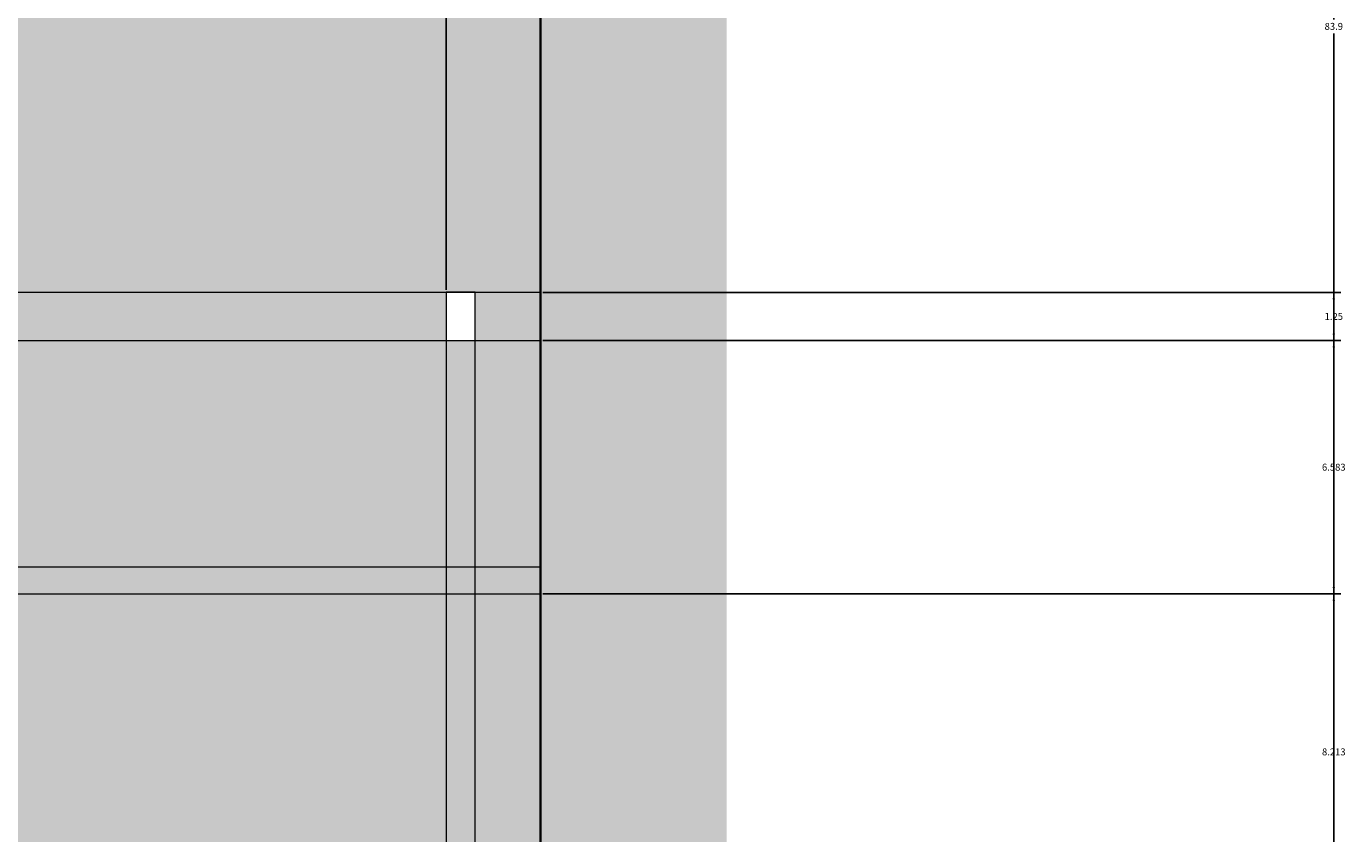
# Model space of a CAD drawing. Units: feet. Extents: x 2695 to 2912, y 795 to 1139.
# Tile 60 of 83: x 2877 to 2912, y 958 to 979. Entities that reach past the tile are written whole.
import ezdxf

# ---------------------------------------------------------------- set-up
doc = ezdxf.new("R2010")
doc.units = ezdxf.units.FT
for name, color, linetype, lineweight in [('A-ANNO-DIMS', 2, 'Continuous', 18), ('A-ELEV', 7, 'Continuous', 35), ('A-ELEV-PATT', 252, 'Continuous', 13), ('A-ELEV-RAIL', 8, 'Continuous', 18)]:
    doc.layers.add(name, color=color, linetype=linetype, lineweight=lineweight)
doc.styles.get("Standard").update_dxf_attribs({"font": 'arial.ttf'})
doc.dimstyles.get("Standard").update_dxf_attribs({"dimtxt": 0.18, "dimasz": 0.18, "dimexe": 0.18, "dimexo": 0.0625, "dimgap": 0.09, "dimtad": 0, "dimtih": 1, "dimtoh": 1, "dimdec": 1, "dimzin": 0, "dimdsep": 46, "dimlunit": 3, "dimtxsty": 'Standard', "dimcen": 0.09, "dimadec": 0, "dimazin": 0, "dimtfac": 1, "dimtdec": 1, "dimtofl": 0, "dimtmove": 0, "dimatfit": 3, "dimfxl": 1, "dimtolj": 1, "dimtzin": 0, "dimarcsym": 0})

# ---------------------------------------------------------------- blocks, each defined once
blk = doc.blocks.new('*D17')
at = {"layer": 'A-ANNO-DIMS', "color": 0, "lineweight": -2, "transparency": 16777216}
for p, q in [((2843.637, 1020.824), (2911.424, 1020.824)), ((2911.244, 1020.644), (2911.244, 979.059)), ((2911.244, 937.111), (2911.244, 978.695)), ((2890.699, 936.931), (2911.424, 936.931))]:
    blk.add_line(p, q, dxfattribs=at)
at = {"layer": 'A-ANNO-DIMS', "color": 0, "transparency": 16777216}
for points in [[(2911.214, 1020.644), (2911.274, 1020.644), (2911.244, 1020.824)], [(2911.214, 937.111), (2911.274, 937.111), (2911.244, 936.931)]]:
    blk.add_solid(points, dxfattribs=at)
at = {"layer": 'Defpoints', "color": 0, "transparency": 16777216}
for p in [(2843.575, 1020.824), (2911.244, 1020.824), (2890.636, 936.931)]:
    blk.add_point(p, dxfattribs=at)
at = {"layer": 'A-ANNO-DIMS', "color": 0, "transparency": 16777216, "insert": (2911.244, 978.877), "char_height": 0.18, "attachment_point": 5}
blk.add_mtext('\\A1;83.9', dxfattribs=at)
blk = doc.blocks.new('*D50')
at = {"layer": 'A-ANNO-DIMS', "color": 0, "lineweight": -2, "transparency": 16777216}
for p, q in [((2810.041, 972.03), (2810.041, 1138.886)), ((2888.188, 972.03), (2888.188, 1138.886)), ((2810.221, 1138.706), (2848.721, 1138.706)), ((2888.008, 1138.706), (2849.508, 1138.706))]:
    blk.add_line(p, q, dxfattribs=at)
at = {"layer": 'A-ANNO-DIMS', "color": 0, "transparency": 16777216}
for points in [[(2810.221, 1138.736), (2810.221, 1138.676), (2810.041, 1138.706)], [(2888.008, 1138.736), (2888.008, 1138.676), (2888.188, 1138.706)]]:
    blk.add_solid(points, dxfattribs=at)
at = {"layer": 'Defpoints', "color": 0, "transparency": 16777216}
for p in [(2888.188, 1138.706), (2810.041, 971.967), (2888.188, 971.967)]:
    blk.add_point(p, dxfattribs=at)
at = {"layer": 'A-ANNO-DIMS', "color": 0, "transparency": 16777216, "insert": (2849.114, 1138.706), "char_height": 0.18, "attachment_point": 5}
blk.add_mtext('\\A1;78.15', dxfattribs=at)
blk = doc.blocks.new('*D51')
at = {"layer": 'A-ANNO-DIMS', "color": 0, "lineweight": -2, "transparency": 16777216}
for p, q in [((2888.188, 972.03), (2888.188, 1138.886)), ((2890.636, 972.03), (2890.636, 1138.886)), ((2888.368, 1138.706), (2889.017, 1138.706)), ((2890.456, 1138.706), (2889.808, 1138.706))]:
    blk.add_line(p, q, dxfattribs=at)
at = {"layer": 'A-ANNO-DIMS', "color": 0, "transparency": 16777216}
for points in [[(2888.368, 1138.736), (2888.368, 1138.676), (2888.188, 1138.706)], [(2890.456, 1138.736), (2890.456, 1138.676), (2890.636, 1138.706)]]:
    blk.add_solid(points, dxfattribs=at)
at = {"layer": 'Defpoints', "color": 0, "transparency": 16777216}
for p in [(2890.636, 1138.706), (2888.188, 971.967), (2890.636, 971.967)]:
    blk.add_point(p, dxfattribs=at)
at = {"layer": 'A-ANNO-DIMS', "color": 0, "transparency": 16777216, "insert": (2889.412, 1138.706), "char_height": 0.18, "attachment_point": 5}
blk.add_mtext('\\A1;2.448', dxfattribs=at)
blk = doc.blocks.new('*D57')
at = {"layer": 'A-ANNO-DIMS', "color": 0, "lineweight": -2, "transparency": 16777216}
for p, q in [((2890.699, 964.133), (2911.424, 964.133)), ((2911.244, 963.953), (2911.244, 960.208)), ((2911.244, 956.1), (2911.244, 959.845)), ((2890.699, 955.92), (2911.424, 955.92))]:
    blk.add_line(p, q, dxfattribs=at)
at = {"layer": 'A-ANNO-DIMS', "color": 0, "transparency": 16777216}
for points in [[(2911.214, 963.953), (2911.274, 963.953), (2911.244, 964.133)], [(2911.214, 956.1), (2911.274, 956.1), (2911.244, 955.92)]]:
    blk.add_solid(points, dxfattribs=at)
at = {"layer": 'Defpoints', "color": 0, "transparency": 16777216}
for p in [(2890.636, 964.133), (2911.244, 964.133), (2890.636, 955.92)]:
    blk.add_point(p, dxfattribs=at)
at = {"layer": 'A-ANNO-DIMS', "color": 0, "transparency": 16777216, "insert": (2911.244, 960.027), "char_height": 0.18, "attachment_point": 5}
blk.add_mtext('\\A1;8.213', dxfattribs=at)
blk = doc.blocks.new('*D58')
at = {"layer": 'A-ANNO-DIMS', "color": 0, "lineweight": -2, "transparency": 16777216}
for p, q in [((2890.699, 970.716), (2911.424, 970.716)), ((2911.244, 970.536), (2911.244, 967.606)), ((2911.244, 964.313), (2911.244, 967.242)), ((2890.699, 964.133), (2911.424, 964.133))]:
    blk.add_line(p, q, dxfattribs=at)
at = {"layer": 'A-ANNO-DIMS', "color": 0, "transparency": 16777216}
for points in [[(2911.214, 970.536), (2911.274, 970.536), (2911.244, 970.716)], [(2911.214, 964.313), (2911.274, 964.313), (2911.244, 964.133)]]:
    blk.add_solid(points, dxfattribs=at)
at = {"layer": 'Defpoints', "color": 0, "transparency": 16777216}
for p in [(2890.636, 970.716), (2911.244, 970.716), (2890.636, 964.133)]:
    blk.add_point(p, dxfattribs=at)
at = {"layer": 'A-ANNO-DIMS', "color": 0, "transparency": 16777216, "insert": (2911.244, 967.424), "char_height": 0.18, "attachment_point": 5}
blk.add_mtext('\\A1;6.583', dxfattribs=at)
blk = doc.blocks.new('*D59')
at = {"layer": 'A-ANNO-DIMS', "color": 0, "lineweight": -2, "transparency": 16777216}
for p, q in [((2890.699, 971.967), (2911.424, 971.967)), ((2911.244, 971.787), (2911.244, 971.523)), ((2911.244, 970.896), (2911.244, 971.16)), ((2890.699, 970.716), (2911.424, 970.716))]:
    blk.add_line(p, q, dxfattribs=at)
at = {"layer": 'A-ANNO-DIMS', "color": 0, "transparency": 16777216}
for points in [[(2911.214, 971.787), (2911.274, 971.787), (2911.244, 971.967)], [(2911.214, 970.896), (2911.274, 970.896), (2911.244, 970.716)]]:
    blk.add_solid(points, dxfattribs=at)
at = {"layer": 'Defpoints', "color": 0, "transparency": 16777216}
for p in [(2890.636, 971.967), (2911.244, 971.967), (2890.636, 970.716)]:
    blk.add_point(p, dxfattribs=at)
at = {"layer": 'A-ANNO-DIMS', "color": 0, "transparency": 16777216, "insert": (2911.244, 971.341), "char_height": 0.18, "attachment_point": 5}
blk.add_mtext('\\A1;1.25', dxfattribs=at)

msp = doc.modelspace()

# ---------------------------------------------------------------- hatches: boundary and pattern name
at = {"layer": 'A-ELEV-PATT'}
h = msp.add_hatch(color=256, dxfattribs=at)
h.set_gradient(color1=(147, 149, 152), color2=(147, 149, 152), tint=1)
h.paths.add_polyline_path([(2770.6361, 1118.4096), (2710.6361, 1118.4096), (2710.6361, 1062.9306), (2770.6361, 1062.9306)])
h.paths.add_polyline_path([(2890.6361, 1103.3378), (2770.6361, 1103.3378), (2770.6361, 1062.9306), (2890.6361, 1062.9306)])
h.paths.add_polyline_path([(2730.7081, 1048.1052), (2755.1125, 1048.1052), (2755.1125, 936.9306), (2770.6361, 936.9306), (2770.6361, 1050.3105), (2715.8852, 1050.3105), (2715.8852, 936.9306), (2730.7081, 936.9306)])
h.paths.add_polyline_path([(2890.6361, 1050.3105), (2770.6361, 1050.3105), (2770.6361, 971.9673), (2778.0341, 971.9673), (2778.0341, 1020.8235), (2843.575, 1020.8235), (2843.575, 971.9673), (2890.6361, 971.9673)])
h.paths.add_polyline_path([(2888.1882, 970.7156), (2843.575, 970.7156), (2843.575, 964.8267), (2888.1882, 964.8267)])
h.paths.add_polyline_path([(2888.1882, 964.1328), (2843.575, 964.1328), (2843.575, 956.614), (2888.1882, 956.614)])
h.paths.add_polyline_path([(2888.1882, 955.9202), (2843.575, 955.9202), (2843.575, 949.2892), (2888.1882, 949.2892)])
h.paths.add_polyline_path([(2888.1882, 948.5954), (2843.575, 948.5954), (2843.575, 941.3507), (2888.1882, 941.3507)])
h.paths.add_polyline_path([(2888.1882, 940.6569), (2843.575, 940.6569), (2843.575, 936.9306), (2888.1882, 936.9306)])
h.paths.add_polyline_path([(2890.6361, 970.7156), (2888.9368, 970.7156), (2888.9368, 964.8267), (2890.6361, 964.8267)])
h.paths.add_polyline_path([(2890.6361, 964.1328), (2888.9368, 964.1328), (2888.9368, 956.614), (2890.6361, 956.614)])
h.paths.add_polyline_path([(2890.6361, 955.9202), (2888.9368, 955.9202), (2888.9368, 949.2892), (2890.6361, 949.2892)])
h.paths.add_polyline_path([(2890.6361, 940.6569), (2888.9368, 940.6569), (2888.9368, 936.9306), (2890.6361, 936.9306)])
h.paths.add_polyline_path([(2890.6361, 948.5954), (2888.9368, 948.5954), (2888.9368, 941.3507), (2890.6361, 941.3507)])
h.paths.add_polyline_path([(2772.5216, 970.7156), (2770.6361, 970.7156), (2770.6361, 964.8267), (2772.5216, 964.8267)])
h.paths.add_polyline_path([(2772.5216, 964.1328), (2770.6361, 964.1328), (2770.6361, 956.614), (2772.5216, 956.614)])
h.paths.add_polyline_path([(2772.5216, 955.9202), (2770.6361, 955.9202), (2770.6361, 949.2892), (2772.5216, 949.2892)])
h.paths.add_polyline_path([(2772.5216, 948.5954), (2770.6361, 948.5954), (2770.6361, 941.3507), (2772.5216, 941.3507)])
h.paths.add_polyline_path([(2772.5216, 940.6569), (2770.6361, 940.6569), (2770.6361, 936.9306), (2772.5216, 936.9306)])
h.paths.add_polyline_path([(2778.0341, 940.6569), (2773.2702, 940.6569), (2773.2702, 936.9306), (2778.0341, 936.9306)])
h.paths.add_polyline_path([(2778.0341, 970.7156), (2773.2702, 970.7156), (2773.2702, 964.8267), (2778.0341, 964.8267)])
h.paths.add_polyline_path([(2778.0341, 964.1328), (2773.2702, 964.1328), (2773.2702, 956.614), (2778.0341, 956.614)])
h.paths.add_polyline_path([(2778.0341, 955.9202), (2773.2702, 955.9202), (2773.2702, 949.2892), (2778.0341, 949.2892)])
h.paths.add_polyline_path([(2778.0341, 948.5954), (2773.2702, 948.5954), (2773.2702, 941.3507), (2778.0341, 941.3507)])
h.paths.add_polyline_path([(2810.0407, 940.6569), (2780.0341, 940.6569), (2780.0341, 936.9306), (2810.0407, 936.9306)])
h.paths.add_polyline_path([(2890.6361, 924.3105), (2770.6361, 924.3105), (2770.6361, 810.9306), (2773.5029, 810.9306), (2773.5029, 905.5143), (2805.9398, 905.5143), (2838.3767, 905.5143), (2838.3767, 810.9306), (2890.6361, 810.9306)])
h = msp.add_hatch(color=256, dxfattribs=at)
h.set_gradient(color1=(255, 255, 255), tint=1)
h.paths.add_polyline_path([(2895.4694, 1107.8588), (2890.6361, 1107.8588), (2890.6361, 810.9306), (2895.4694, 810.9306)])
h = msp.add_hatch(color=256, dxfattribs=at)
h.set_gradient(color1=(255, 255, 255), tint=1)
h.paths.add_polyline_path([(2890.6361, 1050.3105), (2881.9484, 1050.3105), (2881.9484, 971.9673), (2890.6361, 971.9673)])
h.paths.add_polyline_path([(2888.1882, 970.7156), (2881.9484, 970.7156), (2881.9484, 964.8267), (2888.1882, 964.8267)])
h.paths.add_polyline_path([(2890.6361, 970.7156), (2888.9368, 970.7156), (2888.9368, 964.8267), (2890.6361, 964.8267)])
h.paths.add_polyline_path([(2888.1882, 964.1328), (2881.9484, 964.1328), (2881.9484, 956.614), (2888.1882, 956.614)])
h.paths.add_polyline_path([(2890.6361, 964.1328), (2888.9368, 964.1328), (2888.9368, 956.614), (2890.6361, 956.614)])
h.paths.add_polyline_path([(2888.1882, 955.9202), (2881.9484, 955.9202), (2881.9484, 949.2892), (2888.1882, 949.2892)])
h.paths.add_polyline_path([(2890.6361, 955.9202), (2888.9368, 955.9202), (2888.9368, 949.2892), (2890.6361, 949.2892)])
h.paths.add_polyline_path([(2888.1882, 948.5954), (2881.9484, 948.5954), (2881.9484, 941.3507), (2888.1882, 941.3507)])
h.paths.add_polyline_path([(2890.6361, 948.5954), (2888.9368, 948.5954), (2888.9368, 941.3507), (2890.6361, 941.3507)])
h.paths.add_polyline_path([(2888.1882, 940.6569), (2881.9484, 940.6569), (2881.9484, 936.9306), (2888.1882, 936.9306)])
h = msp.add_hatch(color=256, dxfattribs=at)
h.set_gradient(color2=(0, 0, 0), tint=1)
h.paths.add_polyline_path([(2772.5216, 971.9673), (2770.6361, 971.9673), (2770.6361, 970.7156), (2772.5216, 970.7156)])
h.paths.add_polyline_path([(2773.2702, 971.9673), (2772.5216, 971.9673), (2772.5216, 970.7156), (2773.2702, 970.7156)])
h.paths.add_polyline_path([(2778.0341, 971.9673), (2773.2702, 971.9673), (2773.2702, 970.7156), (2778.0341, 970.7156)])
h.paths.add_polyline_path([(2780.0341, 971.9673), (2778.0341, 971.9673), (2778.0341, 970.7156), (2780.0341, 970.7156)])
h.paths.add_polyline_path([(2841.575, 971.9673), (2780.0341, 971.9673), (2780.0341, 970.7156), (2841.575, 970.7156)])
h.paths.add_polyline_path([(2843.575, 971.9673), (2841.575, 971.9673), (2841.575, 970.7156), (2843.575, 970.7156)])
h.paths.add_polyline_path([(2888.1882, 971.9673), (2843.575, 971.9673), (2843.575, 970.7156), (2888.1882, 970.7156)])
h.paths.add_polyline_path([(2888.9368, 971.9673), (2888.1882, 971.9673), (2888.1882, 970.7156), (2888.9368, 970.7156)], flags=17)
h.paths.add_polyline_path([(2890.6361, 971.9673), (2888.9368, 971.9673), (2888.9368, 970.7156), (2890.6361, 970.7156)])
h.paths.add_polyline_path([(2888.9368, 971.9673), (2888.1882, 971.9673), (2888.1882, 964.8267), (2888.9368, 964.8267)])
h.paths.add_polyline_path([(2888.9368, 964.8267), (2888.1882, 964.8267), (2888.1882, 964.1328), (2888.9368, 964.1328)])
h.paths.add_polyline_path([(2890.6361, 964.8267), (2888.9368, 964.8267), (2888.9368, 964.1328), (2890.6361, 964.1328)])
h.paths.add_polyline_path([(2888.1882, 964.8267), (2770.6361, 964.8267), (2770.6361, 964.1328), (2888.1882, 964.1328)])
h.paths.add_polyline_path([(2888.9368, 964.1328), (2888.1882, 964.1328), (2888.1882, 936.9306), (2888.9368, 936.9306)])
h.paths.add_polyline_path([(2890.6361, 956.614), (2888.9368, 956.614), (2888.9368, 955.9202), (2890.6361, 955.9202)])
h.paths.add_polyline_path([(2888.1882, 956.614), (2770.6361, 956.614), (2770.6361, 955.9202), (2888.1882, 955.9202)])
h.paths.add_polyline_path([(2890.6361, 949.2892), (2888.9368, 949.2892), (2888.9368, 948.5954), (2890.6361, 948.5954)])
h.paths.add_polyline_path([(2888.1882, 949.2892), (2770.6361, 949.2892), (2770.6361, 948.5954), (2888.1882, 948.5954)])
h.paths.add_polyline_path([(2890.6361, 941.3507), (2888.9368, 941.3507), (2888.9368, 940.6569), (2890.6361, 940.6569)])
h.paths.add_polyline_path([(2888.1882, 941.3507), (2770.6361, 941.3507), (2770.6361, 940.6569), (2888.1882, 940.6569)])
h.paths.add_polyline_path([(2773.2702, 970.7156), (2772.5216, 970.7156), (2772.5216, 964.8267), (2773.2702, 964.8267)])
h.paths.add_polyline_path([(2773.2702, 964.1328), (2772.5216, 964.1328), (2772.5216, 956.614), (2773.2702, 956.614)])
h.paths.add_polyline_path([(2773.2702, 955.9202), (2772.5216, 955.9202), (2772.5216, 936.9306), (2773.2702, 936.9306)])
h.paths.add_polyline_path([(2810.7893, 970.7156), (2810.0407, 970.7156), (2810.0407, 964.8267), (2810.7893, 964.8267)], flags=17)
h.paths.add_polyline_path([(2810.7893, 964.1328), (2810.0407, 964.1328), (2810.0407, 956.614), (2810.7893, 956.614)], flags=17)
h.paths.add_polyline_path([(2810.7893, 955.9202), (2810.0407, 955.9202), (2810.0407, 949.2892), (2810.7893, 949.2892)], flags=17)
h.paths.add_polyline_path([(2810.7893, 971.9673), (2810.0407, 971.9673), (2810.0407, 941.3507), (2810.7893, 941.3507)])
h.paths.add_polyline_path([(2810.7893, 940.6569), (2810.0407, 940.6569), (2810.0407, 936.9306), (2810.7893, 936.9306)])
h.paths.add_polyline_path([(2780.0341, 1018.8235), (2841.575, 1018.8235), (2841.575, 971.9673), (2843.575, 971.9673), (2843.575, 1020.8235), (2778.0341, 1020.8235), (2778.0341, 971.9673), (2780.0341, 971.9673)])
h.paths.add_polyline_path([(2780.0341, 970.7156), (2778.0341, 970.7156), (2778.0341, 964.8267), (2780.0341, 964.8267)])
h.paths.add_polyline_path([(2780.0341, 964.1328), (2778.0341, 964.1328), (2778.0341, 956.614), (2780.0341, 956.614)])
h.paths.add_polyline_path([(2780.0341, 955.9202), (2778.0341, 955.9202), (2778.0341, 949.2892), (2780.0341, 949.2892)])
h.paths.add_polyline_path([(2780.0341, 948.5954), (2778.0341, 948.5954), (2778.0341, 941.3507), (2780.0341, 941.3507)])
h.paths.add_polyline_path([(2780.0341, 940.6569), (2778.0341, 940.6569), (2778.0341, 936.9306), (2780.0341, 936.9306)])
h.paths.add_polyline_path([(2843.575, 940.6569), (2841.575, 940.6569), (2841.575, 936.9306), (2843.575, 936.9306)])
h.paths.add_polyline_path([(2843.575, 948.5954), (2841.575, 948.5954), (2841.575, 941.3507), (2843.575, 941.3507)])
h.paths.add_polyline_path([(2843.575, 970.7156), (2841.575, 970.7156), (2841.575, 964.8267), (2843.575, 964.8267)])
h.paths.add_polyline_path([(2843.575, 964.1328), (2841.575, 964.1328), (2841.575, 956.614), (2843.575, 956.614)])
h.paths.add_polyline_path([(2843.575, 955.9202), (2841.575, 955.9202), (2841.575, 949.2892), (2843.575, 949.2892)])
h.paths.add_polyline_path([(2805.0538, 874.1057), (2803.9681, 874.1057), (2803.9681, 846.2857), (2805.0538, 846.2857)])
h.paths.add_polyline_path([(2758.1515, 902.577), (2724.1893, 902.577), (2724.1893, 874.8571), (2758.1515, 874.8571)])
h.paths.add_polyline_path([(2726.1893, 900.577), (2756.1515, 900.577), (2756.1515, 876.8571), (2726.1893, 876.8571)], flags=16)
h.paths.add_polyline_path([(2740.7302, 900.577), (2741.6105, 900.577), (2741.6105, 876.8571), (2740.7302, 876.8571)], flags=0)

# ---------------------------------------------------------------- linework, layer by layer
at = {"layer": 'A-ELEV'}
for p, q in [((2890.6361, 810.9306), (2890.6361, 1107.8588)), ((2890.6361, 1062.9306), (2890.6361, 810.9306))]:
    msp.add_line(p, q, dxfattribs=at)
at = {"layer": 'A-ELEV-RAIL'}
msp.add_line((2770.6361, 971.9673), (2890.6361, 971.9673), dxfattribs=at)
for points in [[(2888.9368, 971.9673), (2888.1882, 971.9673), (2888.1882, 936.9306), (2888.9368, 936.9306)], [(2770.6361, 964.1328), (2890.6361, 964.1328), (2890.6361, 964.8267), (2770.6361, 964.8267)]]:
    msp.add_lwpolyline(points, close=True, dxfattribs=at)
msp.add_lwpolyline([(2770.6361, 970.7156), (2890.6361, 970.7156)], dxfattribs=at)

# ---------------------------------------------------------------- dimensions: what is measured, and where the dimension line sits
at = {"layer": 'A-ANNO-DIMS'}
for base, p1, p2, override, picture, middle in [((2888.1882, 1138.7056), (2810.0407, 971.9673), (2888.1882, 971.9673), {"dimdec": 2, "dimlfac": 1, "dimrnd": 0, "dimzin": 0, "dimdsep": 46, "dimlunit": 2}, '*D50', (2849.1144, 1138.7056)), ((2890.6361, 1138.7056), (2888.1882, 971.9673), (2890.6361, 971.9673), {"dimdec": 3, "dimlfac": 1, "dimrnd": 0, "dimzin": 0, "dimdsep": 46, "dimlunit": 2}, '*D51', (2889.4121, 1138.7056))]:
    dim = msp.add_linear_dim(base=base, p1=p1, p2=p2, dimstyle='Standard', override=override, dxfattribs=at)
    dim.commit()
    dim.dimension.update_dxf_attribs({"geometry": picture, "text_midpoint": middle})
for base, p1, p2, override, picture, middle in [((2911.2444, 1020.8235), (2890.6361, 936.9306), (2843.575, 1020.8235), {"dimdec": 1, "dimlfac": 1, "dimrnd": 0, "dimzin": 0, "dimdsep": 46, "dimlunit": 2}, '*D17', (2911.2444, 978.877)), ((2911.2444, 971.9673), (2890.6361, 970.7156), (2890.6361, 971.9673), {"dimdec": 2, "dimlfac": 1, "dimrnd": 0, "dimzin": 0, "dimdsep": 46, "dimlunit": 2}, '*D59', (2911.2444, 971.3414)), ((2911.2444, 970.7156), (2890.6361, 964.1328), (2890.6361, 970.7156), {"dimdec": 3, "dimlfac": 1, "dimrnd": 0, "dimzin": 0, "dimdsep": 46, "dimlunit": 2}, '*D58', (2911.2444, 967.4242)), ((2911.2444, 964.1328), (2890.6361, 955.9202), (2890.6361, 964.1328), {"dimdec": 3, "dimlfac": 1, "dimrnd": 0, "dimzin": 0, "dimdsep": 46, "dimlunit": 2}, '*D57', (2911.2444, 960.0265))]:
    dim = msp.add_linear_dim(base=base, p1=p1, p2=p2, angle=90, dimstyle='Standard', override=override, dxfattribs=at)
    dim.commit()
    dim.dimension.update_dxf_attribs({"geometry": picture, "text_midpoint": middle})

doc.saveas('drawing.dxf')
